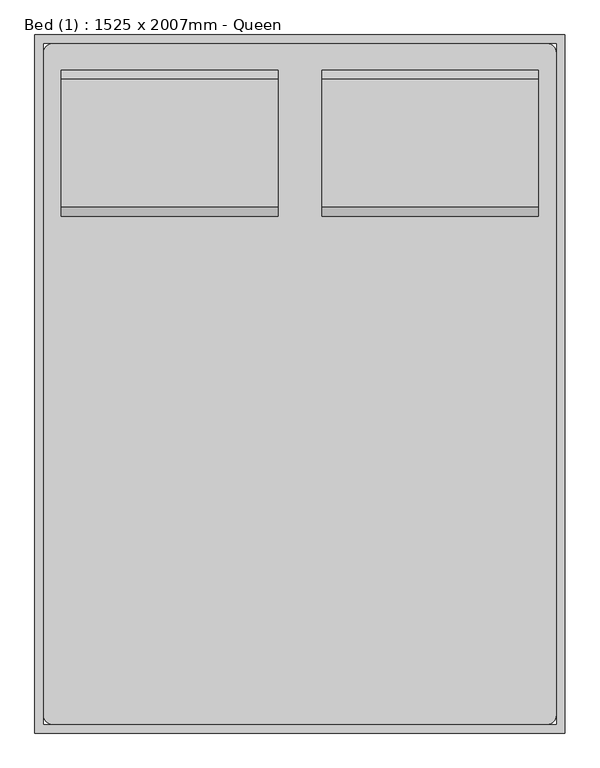
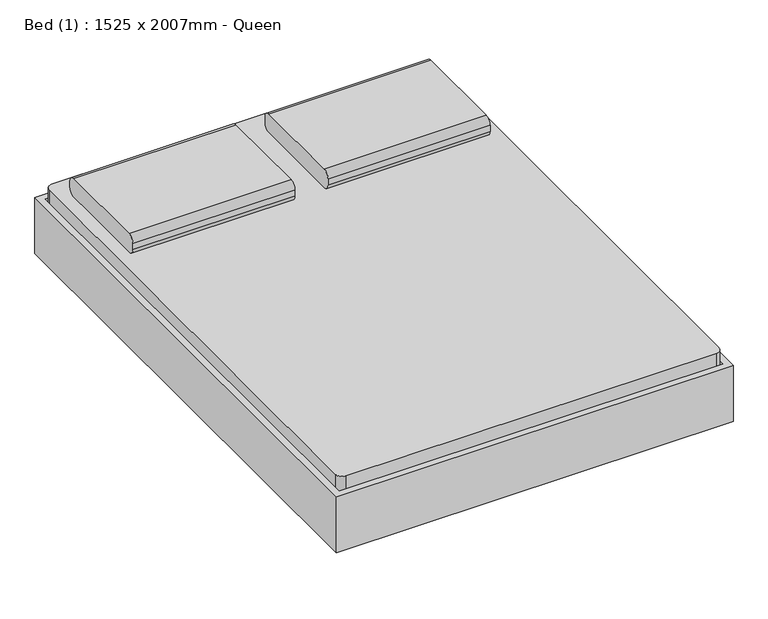
"""IFC4 building model written with IfcOpenShell, lengths in millimetres: furniture geometry, Bed (1) : 1525 x 2007mm - Queen."""

from ifc_helpers import new_model, si_unit, point, frame, frame_2d, origin, place, context, project, spatial, polyline, circle_curve, trimmed, segment, composite_curve, outline, extrude, source, transform, mapped, element, save
from ifc_brep_helpers import plane_surface, cylinder_surface, revolved_surface, advanced_brep


def bed_1_1525_x_2007mm_queen_eef227c3(model_context):
    return source(origin(), model_context, "Body", "SolidModel", [
        advanced_brep(
        [(-397.947541, -933.1295082, 196.85), (-397.947541, -933.1295082, 177.8), (-397.947541, -1009.3295082, 177.8), (-397.947541, -1009.3295082, 196.85), (-335.0113525, -933.1295082, 196.85), (-347.147541, -933.1295082, 177.8), (-347.147541, -1009.3295082, 177.8), (-335.0113525, -1009.3295082, 196.85), (-253.8115092, -933.1295082, 22.716374), (-271.0766725, -933.1295082, 14.6654962), (-271.0766725, -1009.3295082, 14.6654962), (-253.8115092, -1009.3295082, 22.716374), (-248.0564547, -933.1295082, 0.0), (-248.0564547, -933.1295082, 19.05), (-248.0564547, -1009.3295082, 0.0), (-248.0564547, -1009.3295082, 19.05), (-169.4439489, -933.1295082, 19.05), (-169.4439489, -933.1295082, 0.0), (-169.4439489, -1009.3295082, 0.0), (-169.4439489, -1009.3295082, 19.05), (-156.7439489, -933.1295082, 3.4029547), (-166.2689489, -933.1295082, 19.9007387), (-156.7439489, -1009.3295082, 3.4029547), (-166.2689489, -1009.3295082, 19.9007387), (-101.7513357, -933.1295082, 57.15), (-96.6469036, -933.1295082, 38.1), (-96.6469036, -1009.3295082, 38.1), (-101.7513357, -1009.3295082, 57.15), (780.0562537, -933.1295082, 57.15), (774.9518216, -933.1295082, 38.1), (774.9518216, -1009.3295082, 38.1), (780.0562537, -1009.3295082, 57.15), (844.5738669, -933.1295082, 19.9007387), (835.0488669, -933.1295082, 3.4029547), (835.0488669, -1009.3295082, 3.4029547), (844.5738669, -1009.3295082, 19.9007387), (847.7488669, -933.1295082, 0.0), (847.7488669, -933.1295082, 19.05), (847.7488669, -1009.3295082, 0.0), (847.7488669, -1009.3295082, 19.05), (926.3613728, -933.1295082, 19.05), (926.3613728, -933.1295082, 0.0), (926.3613728, -1009.3295082, 0.0), (926.3613728, -1009.3295082, 19.05), (949.3815906, -933.1295082, 14.6654962), (932.1164272, -933.1295082, 22.716374), (949.3815906, -1009.3295082, 14.6654962), (932.1164272, -1009.3295082, 22.716374), (1013.3162705, -933.1295082, 196.85), (1025.452459, -933.1295082, 177.8), (1025.452459, -1009.3295082, 177.8), (1013.3162705, -1009.3295082, 196.85), (1076.252459, -933.1295082, 196.85), (1076.252459, -1009.3295082, 196.85), (1076.252459, -1009.3295082, 177.8), (1076.252459, -933.1295082, 177.8)],
        [
            (0, 1),
            (1, 2),
            (2, 3),
            (3, 0),
            (0, 4),
            (4, 5),
            (5, 1),
            (5, 6),
            (6, 2),
            (6, 7),
            (7, 3),
            (7, 4),
            (4, 8),
            (8, 9),
            (9, 5),
            (9, 10),
            (10, 6),
            (10, 11),
            (11, 7),
            (11, 8),
            (12, 9, circle_curve(frame((-248.0564547, -933.1295082, 25.4), z_axis=(0.0, 1.0, 0.0), x_axis=(-0.906307787036664, 0.0, -0.4226182617406693)), 25.4)),
            (8, 13, circle_curve(frame((-248.0564547, -933.1295082, 25.4), z_axis=(0.0, -1.0, 0.0), x_axis=(-0.906307787036664, 0.0, -0.4226182617406693)), 6.35)),
            (13, 12),
            (14, 10, circle_curve(frame((-248.0564547, -1009.3295082, 25.4), z_axis=(0.0, 1.0, 0.0), x_axis=(-0.906307787036664, 0.0, -0.4226182617406693)), 25.4)),
            (12, 14),
            (15, 11, circle_curve(frame((-248.0564547, -1009.3295082, 25.4), z_axis=(0.0, 1.0, 0.0), x_axis=(-0.906307787036664, 0.0, -0.4226182617406693)), 6.35)),
            (14, 15),
            (15, 13),
            (13, 16),
            (16, 17),
            (17, 12),
            (17, 18),
            (18, 14),
            (18, 19),
            (19, 15),
            (19, 16),
            (20, 17, circle_curve(frame((-169.4439489, -933.1295082, 25.4), z_axis=(0.0, 1.0, 0.0), x_axis=(0.0, 0.0, -1.0)), 25.4)),
            (16, 21, circle_curve(frame((-169.4439489, -933.1295082, 25.4), z_axis=(0.0, -1.0, 0.0), x_axis=(0.0, 0.0, -1.0)), 6.35)),
            (21, 20),
            (22, 18, circle_curve(frame((-169.4439489, -1009.3295082, 25.4), z_axis=(0.0, 1.0, 0.0), x_axis=(0.0, 0.0, -1.0)), 25.4)),
            (20, 22),
            (23, 19, circle_curve(frame((-169.4439489, -1009.3295082, 25.4), z_axis=(0.0, 1.0, 0.0), x_axis=(0.0, 0.0, -1.0)), 6.35)),
            (22, 23),
            (23, 21),
            (21, 24),
            (24, 25),
            (25, 20),
            (25, 26),
            (26, 22),
            (26, 27),
            (27, 23),
            (27, 24),
            (24, 28),
            (28, 29),
            (29, 25),
            (29, 30),
            (30, 26),
            (30, 31),
            (31, 27),
            (31, 28),
            (28, 32),
            (32, 33),
            (33, 29),
            (33, 34),
            (34, 30),
            (34, 35),
            (35, 31),
            (35, 32),
            (36, 33, circle_curve(frame((847.7488669, -933.1295082, 25.4), z_axis=(0.0, 1.0, 0.0), x_axis=(-0.5000000000000533, 0.0, -0.866025403784408)), 25.4)),
            (32, 37, circle_curve(frame((847.7488669, -933.1295082, 25.4), z_axis=(0.0, -1.0, 0.0), x_axis=(-0.5000000000000533, 0.0, -0.866025403784408)), 6.35)),
            (37, 36),
            (38, 34, circle_curve(frame((847.7488669, -1009.3295082, 25.4), z_axis=(0.0, 1.0, 0.0), x_axis=(-0.5000000000000533, 0.0, -0.866025403784408)), 25.4)),
            (36, 38),
            (39, 35, circle_curve(frame((847.7488669, -1009.3295082, 25.4), z_axis=(0.0, 1.0, 0.0), x_axis=(-0.5000000000000533, 0.0, -0.866025403784408)), 6.35)),
            (38, 39),
            (39, 37),
            (37, 40),
            (40, 41),
            (41, 36),
            (41, 42),
            (42, 38),
            (42, 43),
            (43, 39),
            (43, 40),
            (44, 41, circle_curve(frame((926.3613728, -933.1295082, 25.4), z_axis=(0.0, 1.0, 0.0), x_axis=(0.0, 0.0, -1.0)), 25.4)),
            (40, 45, circle_curve(frame((926.3613728, -933.1295082, 25.4), z_axis=(0.0, -1.0, 0.0), x_axis=(0.0, 0.0, -1.0)), 6.35)),
            (45, 44),
            (46, 42, circle_curve(frame((926.3613728, -1009.3295082, 25.4), z_axis=(0.0, 1.0, 0.0), x_axis=(0.0, 0.0, -1.0)), 25.4)),
            (44, 46),
            (47, 43, circle_curve(frame((926.3613728, -1009.3295082, 25.4), z_axis=(0.0, 1.0, 0.0), x_axis=(0.0, 0.0, -1.0)), 6.35)),
            (46, 47),
            (47, 45),
            (45, 48),
            (48, 49),
            (49, 44),
            (49, 50),
            (50, 46),
            (50, 51),
            (51, 47),
            (51, 48),
            (52, 53),
            (53, 54),
            (54, 55),
            (55, 52),
            (48, 52),
            (55, 49),
            (54, 50),
            (53, 51),
        ],
        [
            plane_surface(frame((-397.947541, -1237.9295082, -127.5947323), z_axis=(-1.0, 0.0, 0.0), x_axis=(0.0, 1.0, 0.0))),
            plane_surface(frame((-397.947541, -933.1295082, 196.85), z_axis=(0.0, 1.0, 0.0), x_axis=(1.0, 0.0, 0.0))),
            plane_surface(frame((-397.947541, -933.1295082, 177.8), z_axis=(0.0, 0.0, -1.0), x_axis=(1.0, 0.0, 0.0))),
            plane_surface(frame((-397.947541, -1009.3295082, 177.8), z_axis=(0.0, -1.0, 0.0), x_axis=(1.0, 0.0, 0.0))),
            plane_surface(frame((-397.947541, -1009.3295082, 196.85), z_axis=(0.0, 0.0, 1.0), x_axis=(1.0, 0.0, 0.0))),
            plane_surface(frame((-335.0113525, -933.1295082, 196.85), z_axis=(0.0, 1.0, 0.0), x_axis=(0.42261826174067163, 0.0, -0.9063077870366629))),
            plane_surface(frame((-347.147541, -933.1295082, 177.8), z_axis=(-0.906307787036663, 0.0, -0.4226182617406716), x_axis=(0.4226182617406716, 0.0, -0.906307787036663))),
            plane_surface(frame((-347.147541, -1009.3295082, 177.8), z_axis=(0.0, -1.0000000000000002, 0.0), x_axis=(0.4226182617406714, 0.0, -0.9063077870366631))),
            plane_surface(frame((-335.0113525, -1009.3295082, 196.85), z_axis=(0.906307787036663, 0.0, 0.4226182617406716), x_axis=(0.4226182617406716, 0.0, -0.906307787036663))),
            plane_surface(frame((-248.0564547, -933.1295082, 25.4), z_axis=(0.0, 1.0, 0.0), x_axis=(-0.906307787036664, 0.0, -0.4226182617406693))),
            cylinder_surface(frame((-248.0564547, -1237.9295082, 25.4), z_axis=(0.0, -1.0, 0.0), x_axis=(-0.906307787036664, 0.0, -0.4226182617406693)), 25.4),
            plane_surface(frame((-248.0564547, -1009.3295082, 25.4), z_axis=(0.0, -1.0, 0.0), x_axis=(-0.906307787036664, 0.0, -0.4226182617406693))),
            revolved_surface(polyline([(-253.8115091476828, -1009.3295082, 22.71637403794675), (-253.8115091476828, -933.1295082, 22.71637403794675)]), (-248.0564547, -1237.9295082, 25.4), (0.0, -1.0, 0.0)),
            plane_surface(frame((-248.0564547, -933.1295082, 19.05), z_axis=(0.0, 1.0, 0.0), x_axis=(1.0, 0.0, 0.0))),
            plane_surface(frame((-248.0564547, -933.1295082, 0.0), z_axis=(0.0, 0.0, -1.0), x_axis=(1.0, 0.0, 0.0))),
            plane_surface(frame((-248.0564547, -1009.3295082, 0.0), z_axis=(0.0, -1.0, 0.0), x_axis=(1.0, 0.0, 0.0))),
            plane_surface(frame((-248.0564547, -1009.3295082, 19.05), z_axis=(0.0, 0.0, 1.0), x_axis=(1.0, 0.0, 0.0))),
            plane_surface(frame((-169.4439489, -933.1295082, 25.4), z_axis=(0.0, 1.0, 0.0), x_axis=(0.0, 0.0, -1.0))),
            cylinder_surface(frame((-169.4439489, -1237.9295082, 25.4), z_axis=(0.0, -1.0, 0.0), x_axis=(0.0, 0.0, -1.0)), 25.4),
            plane_surface(frame((-169.4439489, -1009.3295082, 25.4), z_axis=(0.0, -1.0, 0.0), x_axis=(0.0, 0.0, -1.0))),
            revolved_surface(polyline([(-169.4439489, -1009.3295082, 19.049999999999997), (-169.4439489, -933.1295082, 19.049999999999997)]), (-169.4439489, -1237.9295082, 25.4), (0.0, -1.0, 0.0)),
            plane_surface(frame((-166.2689489, -933.1295082, 19.9007387), z_axis=(0.0, 1.0, 0.0), x_axis=(0.8660254037844783, 0.0, 0.4999999999999313))),
            plane_surface(frame((-156.7439489, -933.1295082, 3.4029547), z_axis=(0.499999999999931, 0.0, -0.8660254037844785), x_axis=(0.8660254037844785, 0.0, 0.499999999999931))),
            plane_surface(frame((-156.7439489, -1009.3295082, 3.4029547), z_axis=(0.0, -1.0, 0.0), x_axis=(0.8660254037844787, 0.0, 0.49999999999993067))),
            plane_surface(frame((-166.2689489, -1009.3295082, 19.9007387), z_axis=(-0.4999999999999307, 0.0, 0.8660254037844787), x_axis=(0.8660254037844787, 0.0, 0.4999999999999307))),
            plane_surface(frame((-101.7513357, -933.1295082, 57.15), z_axis=(0.0, 1.0, 0.0), x_axis=(1.0, 0.0, 0.0))),
            plane_surface(frame((-96.6469036, -933.1295082, 38.1), z_axis=(0.0, 0.0, -1.0), x_axis=(1.0, 0.0, 0.0))),
            plane_surface(frame((-96.6469036, -1009.3295082, 38.1), z_axis=(0.0, -1.0, 0.0), x_axis=(1.0, 0.0, 0.0))),
            plane_surface(frame((-101.7513357, -1009.3295082, 57.15), z_axis=(0.0, 0.0, 1.0), x_axis=(1.0, 0.0, 0.0))),
            plane_surface(frame((780.0562537, -933.1295082, 57.15), z_axis=(0.0, 1.0000000000000002, 0.0), x_axis=(0.8660254037844111, 0.0, -0.500000000000048))),
            plane_surface(frame((774.9518216, -933.1295082, 38.1), z_axis=(-0.5000000000000486, 0.0, -0.8660254037844106), x_axis=(0.8660254037844106, 0.0, -0.5000000000000486))),
            plane_surface(frame((774.9518216, -1009.3295082, 38.1), z_axis=(0.0, -1.0000000000000002, 0.0), x_axis=(0.8660254037844111, 0.0, -0.500000000000048))),
            plane_surface(frame((780.0562537, -1009.3295082, 57.15), z_axis=(0.5000000000000487, 0.0, 0.8660254037844106), x_axis=(0.8660254037844106, 0.0, -0.5000000000000487))),
            plane_surface(frame((847.7488669, -933.1295082, 25.4), z_axis=(0.0, 1.0, 0.0), x_axis=(-0.5000000000000533, 0.0, -0.866025403784408))),
            cylinder_surface(frame((847.7488669, -1237.9295082, 25.4), z_axis=(0.0, -1.0, 0.0), x_axis=(-0.5000000000000533, 0.0, -0.866025403784408)), 25.4),
            plane_surface(frame((847.7488669, -1009.3295082, 25.4), z_axis=(0.0, -1.0, 0.0), x_axis=(-0.5000000000000533, 0.0, -0.866025403784408))),
            revolved_surface(polyline([(844.5738668999998, -1009.3295082, 19.90073868596901), (844.5738668999998, -933.1295082, 19.90073868596901)]), (847.7488669, -1237.9295082, 25.4), (0.0, -1.0, 0.0)),
            plane_surface(frame((847.7488669, -933.1295082, 19.05), z_axis=(0.0, 1.0, 0.0), x_axis=(1.0, 0.0, 0.0))),
            plane_surface(frame((847.7488669, -933.1295082, 0.0), z_axis=(0.0, 0.0, -1.0), x_axis=(1.0, 0.0, 0.0))),
            plane_surface(frame((847.7488669, -1009.3295082, 0.0), z_axis=(0.0, -1.0, 0.0), x_axis=(1.0, 0.0, 0.0))),
            plane_surface(frame((847.7488669, -1009.3295082, 19.05), z_axis=(0.0, 0.0, 1.0), x_axis=(1.0, 0.0, 0.0))),
            plane_surface(frame((926.3613728, -933.1295082, 25.4), z_axis=(0.0, 1.0, 0.0), x_axis=(0.0, 0.0, -1.0))),
            cylinder_surface(frame((926.3613728, -1237.9295082, 25.4), z_axis=(0.0, -1.0, 0.0), x_axis=(0.0, 0.0, -1.0)), 25.4),
            plane_surface(frame((926.3613728, -1009.3295082, 25.4), z_axis=(0.0, -1.0, 0.0), x_axis=(0.0, 0.0, -1.0))),
            revolved_surface(polyline([(926.3613728, -1009.3295082, 19.049999999999997), (926.3613728, -933.1295082, 19.049999999999997)]), (926.3613728, -1237.9295082, 25.4), (0.0, -1.0, 0.0)),
            plane_surface(frame((932.1164272, -933.1295082, 22.716374), z_axis=(0.0, 1.0000000000000002, 0.0), x_axis=(0.4226182617405397, 0.0, 0.9063077870367245))),
            plane_surface(frame((949.3815906, -933.1295082, 14.6654962), z_axis=(0.9063077870367244, 0.0, -0.42261826174053974), x_axis=(0.42261826174053974, 0.0, 0.9063077870367244))),
            plane_surface(frame((949.3815906, -1009.3295082, 14.6654962), z_axis=(0.0, -1.0, 0.0), x_axis=(0.4226182617405396, 0.0, 0.9063077870367245))),
            plane_surface(frame((932.1164272, -1009.3295082, 22.716374), z_axis=(-0.9063077870367244, 0.0, 0.42261826174053996), x_axis=(0.42261826174053996, 0.0, 0.9063077870367244))),
            plane_surface(frame((1076.252459, -1237.9295082, -127.5947323), z_axis=(1.0, 0.0, 0.0), x_axis=(0.0, 1.0, 0.0))),
            plane_surface(frame((1013.3162705, -933.1295082, 196.85), z_axis=(0.0, 1.0, 0.0), x_axis=(1.0, 0.0, 0.0))),
            plane_surface(frame((1025.452459, -933.1295082, 177.8), z_axis=(0.0, 0.0, -1.0), x_axis=(1.0, 0.0, 0.0))),
            plane_surface(frame((1025.452459, -1009.3295082, 177.8), z_axis=(0.0, -1.0, 0.0), x_axis=(1.0, 0.0, 0.0))),
            plane_surface(frame((1013.3162705, -1009.3295082, 196.85), z_axis=(0.0, 0.0, 1.0), x_axis=(1.0, 0.0, 0.0))),
        ],
        [
            (0, [[1, 2, 3, 4]]),
            (1, [[-1, 5, 6, 7]]),
            (2, [[-2, -7, 8, 9]]),
            (3, [[-3, -9, 10, 11]]),
            (4, [[-4, -11, 12, -5]]),
            (5, [[-6, 13, 14, 15]]),
            (6, [[-8, -15, 16, 17]]),
            (7, [[-10, -17, 18, 19]]),
            (8, [[-12, -19, 20, -13]]),
            (9, [[21, -14, 22, 23]]),
            (10, [[24, -16, -21, 25]]),
            (11, [[26, -18, -24, 27]]),
            (12, [[-22, -20, -26, 28]]),
            (13, [[-23, 29, 30, 31]]),
            (14, [[-25, -31, 32, 33]]),
            (15, [[-27, -33, 34, 35]]),
            (16, [[-28, -35, 36, -29]]),
            (17, [[37, -30, 38, 39]]),
            (18, [[40, -32, -37, 41]]),
            (19, [[42, -34, -40, 43]]),
            (20, [[-38, -36, -42, 44]]),
            (21, [[-39, 45, 46, 47]]),
            (22, [[-41, -47, 48, 49]]),
            (23, [[-43, -49, 50, 51]]),
            (24, [[-44, -51, 52, -45]]),
            (25, [[-46, 53, 54, 55]]),
            (26, [[-48, -55, 56, 57]]),
            (27, [[-50, -57, 58, 59]]),
            (28, [[-52, -59, 60, -53]]),
            (29, [[-54, 61, 62, 63]]),
            (30, [[-56, -63, 64, 65]]),
            (31, [[-58, -65, 66, 67]]),
            (32, [[-60, -67, 68, -61]]),
            (33, [[69, -62, 70, 71]]),
            (34, [[72, -64, -69, 73]]),
            (35, [[74, -66, -72, 75]]),
            (36, [[-70, -68, -74, 76]]),
            (37, [[-71, 77, 78, 79]]),
            (38, [[-73, -79, 80, 81]]),
            (39, [[-75, -81, 82, 83]]),
            (40, [[-76, -83, 84, -77]]),
            (41, [[85, -78, 86, 87]]),
            (42, [[88, -80, -85, 89]]),
            (43, [[90, -82, -88, 91]]),
            (44, [[-86, -84, -90, 92]]),
            (45, [[-87, 93, 94, 95]]),
            (46, [[-89, -95, 96, 97]]),
            (47, [[-91, -97, 98, 99]]),
            (48, [[-92, -99, 100, -93]]),
            (49, [[101, 102, 103, 104]]),
            (50, [[-94, 105, -104, 106]]),
            (51, [[-96, -106, -103, 107]]),
            (52, [[-98, -107, -102, 108]]),
            (53, [[-100, -108, -101, -105]]),
        ],
    ),
        extrude(outline(composite_curve([segment(polyline([(-372.547541, 743.6704918), (1050.852459, 743.6704918)]), True, "CONTINUOUS"), segment(trimmed(circle_curve(frame_2d((1050.852459, 718.2704918)), 25.4), [point((1050.852459, 743.6704918))], [point((1076.252459, 718.2704918))], False, "CARTESIAN"), True, "CONTINUOUS"), segment(polyline([(1076.252459, 718.2704918), (1076.252459, -1187.1295082)]), True, "CONTINUOUS"), segment(trimmed(circle_curve(frame_2d((1050.852459, -1187.1295082)), 25.4), [point((1076.252459, -1187.1295082))], [point((1050.852459, -1212.5295082))], False, "CARTESIAN"), True, "CONTINUOUS"), segment(polyline([(1050.852459, -1212.5295082), (-372.547541, -1212.5295082)]), True, "CONTINUOUS"), segment(trimmed(circle_curve(frame_2d((-372.547541, -1187.1295082)), 25.4), [point((-372.547541, -1212.5295082))], [point((-397.947541, -1187.1295082))], False, "CARTESIAN"), True, "CONTINUOUS"), segment(polyline([(-397.947541, -1187.1295082), (-397.947541, 718.2704918)]), True, "CONTINUOUS"), segment(trimmed(circle_curve(frame_2d((-372.547541, 718.2704918)), 25.4), [point((-397.947541, 718.2704918))], [point((-372.547541, 743.6704918))], False, "CARTESIAN"), True, "CONTINUOUS")], self_intersect=False)), frame((0.0, 0.0, 203.2), z_axis=(0.0, 0.0, 1.0), x_axis=(1.0, 0.0, 0.0)), (0.0, 0.0, 1.0), 203.2),
        advanced_brep(
        [(-397.6231784, 515.0704918, 177.8), (-397.6231784, 438.8704918, 177.8), (-397.6231784, 438.8704918, 196.85), (-397.6231784, 515.0704918, 196.85), (-346.8231784, 515.0704918, 177.8), (-346.8231784, 438.8704918, 177.8), (-334.6869899, 438.8704918, 196.85), (-334.6869899, 515.0704918, 196.85), (-270.7523099, 515.0704918, 14.6654962), (-270.7523099, 438.8704918, 14.6654962), (-253.4871466, 438.8704918, 22.716374), (-253.4871466, 515.0704918, 22.716374), (-247.7320921, 438.8704918, 0.0), (-247.7320921, 515.0704918, 0.0), (-247.7320921, 438.8704918, 19.05), (-247.7320921, 515.0704918, 19.05), (-169.1195862, 515.0704918, 0.0), (-169.1195862, 438.8704918, 0.0), (-169.1195862, 438.8704918, 19.05), (-169.1195862, 515.0704918, 19.05), (-156.4195862, 438.8704918, 3.4029547), (-156.4195862, 515.0704918, 3.4029547), (-165.9445862, 438.8704918, 19.9007387), (-165.9445862, 515.0704918, 19.9007387), (-96.322541, 515.0704918, 38.1), (-96.322541, 438.8704918, 38.1), (-101.4269731, 438.8704918, 57.15), (-101.4269731, 515.0704918, 57.15), (774.9518216, 515.0704918, 38.1), (774.9518216, 438.8704918, 38.1), (780.0562537, 438.8704918, 57.15), (780.0562537, 515.0704918, 57.15), (835.0488669, 515.0704918, 3.4029547), (835.0488669, 438.8704918, 3.4029547), (844.5738669, 438.8704918, 19.9007387), (844.5738669, 515.0704918, 19.9007387), (847.7488669, 438.8704918, 0.0), (847.7488669, 515.0704918, 0.0), (847.7488669, 438.8704918, 19.05), (847.7488669, 515.0704918, 19.05), (926.3613728, 515.0704918, 0.0), (926.3613728, 438.8704918, 0.0), (926.3613728, 438.8704918, 19.05), (926.3613728, 515.0704918, 19.05), (949.3815906, 438.8704918, 14.6654962), (949.3815906, 515.0704918, 14.6654962), (932.1164272, 438.8704918, 22.716374), (932.1164272, 515.0704918, 22.716374), (1025.452459, 515.0704918, 177.8), (1025.452459, 438.8704918, 177.8), (1013.3162705, 438.8704918, 196.85), (1013.3162705, 515.0704918, 196.85), (1076.252459, 515.0704918, 177.8), (1076.252459, 515.0704918, 196.85), (1076.252459, 438.8704918, 196.85), (1076.252459, 438.8704918, 177.8)],
        [
            (0, 1),
            (1, 2),
            (2, 3),
            (3, 0),
            (0, 4),
            (4, 5),
            (5, 1),
            (5, 6),
            (6, 2),
            (6, 7),
            (7, 3),
            (7, 4),
            (4, 8),
            (8, 9),
            (9, 5),
            (9, 10),
            (10, 6),
            (10, 11),
            (11, 7),
            (11, 8),
            (12, 9, circle_curve(frame((-247.7320921, 438.8704918, 25.4), z_axis=(0.0, 1.0, 0.0), x_axis=(-0.906307787036649, 0.0, -0.4226182617407015)), 25.4)),
            (8, 13, circle_curve(frame((-247.7320921, 515.0704918, 25.4), z_axis=(0.0, -1.0, 0.0), x_axis=(-0.906307787036649, 0.0, -0.4226182617407015)), 25.4)),
            (13, 12),
            (14, 10, circle_curve(frame((-247.7320921, 438.8704918, 25.4), z_axis=(0.0, 1.0, 0.0), x_axis=(-0.906307787036649, 0.0, -0.4226182617407015)), 6.35)),
            (12, 14),
            (15, 11, circle_curve(frame((-247.7320921, 515.0704918, 25.4), z_axis=(0.0, 1.0, 0.0), x_axis=(-0.906307787036649, 0.0, -0.4226182617407015)), 6.35)),
            (14, 15),
            (15, 13),
            (13, 16),
            (16, 17),
            (17, 12),
            (17, 18),
            (18, 14),
            (18, 19),
            (19, 15),
            (19, 16),
            (20, 17, circle_curve(frame((-169.1195862, 438.8704918, 25.4), z_axis=(0.0, 1.0, 0.0), x_axis=(0.0, 0.0, -1.0)), 25.4)),
            (16, 21, circle_curve(frame((-169.1195862, 515.0704918, 25.4), z_axis=(0.0, -1.0, 0.0), x_axis=(0.0, 0.0, -1.0)), 25.4)),
            (21, 20),
            (22, 18, circle_curve(frame((-169.1195862, 438.8704918, 25.4), z_axis=(0.0, 1.0, 0.0), x_axis=(0.0, 0.0, -1.0)), 6.35)),
            (20, 22),
            (23, 19, circle_curve(frame((-169.1195862, 515.0704918, 25.4), z_axis=(0.0, 1.0, 0.0), x_axis=(0.0, 0.0, -1.0)), 6.35)),
            (22, 23),
            (23, 21),
            (21, 24),
            (24, 25),
            (25, 20),
            (25, 26),
            (26, 22),
            (26, 27),
            (27, 23),
            (27, 24),
            (24, 28),
            (28, 29),
            (29, 25),
            (29, 30),
            (30, 26),
            (30, 31),
            (31, 27),
            (31, 28),
            (28, 32),
            (32, 33),
            (33, 29),
            (33, 34),
            (34, 30),
            (34, 35),
            (35, 31),
            (35, 32),
            (36, 33, circle_curve(frame((847.7488669, 438.8704918, 25.4), z_axis=(0.0, 1.0, 0.0), x_axis=(-0.5000000000000449, 0.0, -0.8660254037844127)), 25.4)),
            (32, 37, circle_curve(frame((847.7488669, 515.0704918, 25.4), z_axis=(0.0, -1.0, 0.0), x_axis=(-0.5000000000000449, 0.0, -0.8660254037844127)), 25.4)),
            (37, 36),
            (38, 34, circle_curve(frame((847.7488669, 438.8704918, 25.4), z_axis=(0.0, 1.0, 0.0), x_axis=(-0.5000000000000449, 0.0, -0.8660254037844127)), 6.35)),
            (36, 38),
            (39, 35, circle_curve(frame((847.7488669, 515.0704918, 25.4), z_axis=(0.0, 1.0, 0.0), x_axis=(-0.5000000000000449, 0.0, -0.8660254037844127)), 6.35)),
            (38, 39),
            (39, 37),
            (37, 40),
            (40, 41),
            (41, 36),
            (41, 42),
            (42, 38),
            (42, 43),
            (43, 39),
            (43, 40),
            (44, 41, circle_curve(frame((926.3613728, 438.8704918, 25.4), z_axis=(0.0, 1.0, 0.0), x_axis=(0.0, 0.0, -1.0)), 25.4)),
            (40, 45, circle_curve(frame((926.3613728, 515.0704918, 25.4), z_axis=(0.0, -1.0, 0.0), x_axis=(0.0, 0.0, -1.0)), 25.4)),
            (45, 44),
            (46, 42, circle_curve(frame((926.3613728, 438.8704918, 25.4), z_axis=(0.0, 1.0, 0.0), x_axis=(0.0, 0.0, -1.0)), 6.35)),
            (44, 46),
            (47, 43, circle_curve(frame((926.3613728, 515.0704918, 25.4), z_axis=(0.0, 1.0, 0.0), x_axis=(0.0, 0.0, -1.0)), 6.35)),
            (46, 47),
            (47, 45),
            (45, 48),
            (48, 49),
            (49, 44),
            (49, 50),
            (50, 46),
            (50, 51),
            (51, 47),
            (51, 48),
            (52, 53),
            (53, 54),
            (54, 55),
            (55, 52),
            (48, 52),
            (55, 49),
            (54, 50),
            (53, 51),
        ],
        [
            plane_surface(frame((-397.6231784, 769.0704918, -152.9490627), z_axis=(-1.0, 0.0, 0.0), x_axis=(0.0, 1.0, 0.0))),
            plane_surface(frame((-397.6231784, 515.0704918, 177.8), z_axis=(0.0, 0.0, -1.0), x_axis=(1.0, 0.0, 0.0))),
            plane_surface(frame((-397.6231784, 438.8704918, 177.8), z_axis=(0.0, -1.0, 0.0), x_axis=(1.0, 0.0, 0.0))),
            plane_surface(frame((-397.6231784, 438.8704918, 196.85), z_axis=(0.0, 0.0, 1.0), x_axis=(1.0, 0.0, 0.0))),
            plane_surface(frame((-397.6231784, 515.0704918, 196.85), z_axis=(0.0, 1.0, 0.0), x_axis=(1.0, 0.0, 0.0))),
            plane_surface(frame((-346.8231784, 515.0704918, 177.8), z_axis=(-0.9063077870366485, 0.0, -0.4226182617407029), x_axis=(0.4226182617407029, 0.0, -0.9063077870366485))),
            plane_surface(frame((-346.8231784, 438.8704918, 177.8), z_axis=(0.0, -1.0, 0.0), x_axis=(0.42261826174070266, 0.0, -0.9063077870366485))),
            plane_surface(frame((-334.6869899, 438.8704918, 196.85), z_axis=(0.9063077870366486, 0.0, 0.4226182617407026), x_axis=(0.4226182617407026, 0.0, -0.9063077870366486))),
            plane_surface(frame((-334.6869899, 515.0704918, 196.85), z_axis=(0.0, 1.0, 0.0), x_axis=(0.42261826174070266, 0.0, -0.9063077870366485))),
            cylinder_surface(frame((-247.7320921, 769.0704918, 25.4), z_axis=(0.0, -1.0, 0.0), x_axis=(-0.906307787036649, 0.0, -0.4226182617407015)), 25.4),
            plane_surface(frame((-247.7320921, 438.8704918, 25.4), z_axis=(0.0, -1.0, 0.0), x_axis=(-0.906307787036649, 0.0, -0.4226182617407015))),
            revolved_surface(polyline([(-253.4871465476827, 438.8704918, 22.716374037946544), (-253.4871465476827, 515.0704918, 22.716374037946544)]), (-247.7320921, 769.0704918, 25.4), (0.0, -1.0, 0.0)),
            plane_surface(frame((-247.7320921, 515.0704918, 25.4), z_axis=(0.0, 1.0, 0.0), x_axis=(-0.906307787036649, 0.0, -0.4226182617407015))),
            plane_surface(frame((-247.7320921, 515.0704918, 0.0), z_axis=(0.0, 0.0, -1.0), x_axis=(1.0, 0.0, 0.0))),
            plane_surface(frame((-247.7320921, 438.8704918, 0.0), z_axis=(0.0, -1.0, 0.0), x_axis=(1.0, 0.0, 0.0))),
            plane_surface(frame((-247.7320921, 438.8704918, 19.05), z_axis=(0.0, 0.0, 1.0), x_axis=(1.0, 0.0, 0.0))),
            plane_surface(frame((-247.7320921, 515.0704918, 19.05), z_axis=(0.0, 1.0, 0.0), x_axis=(1.0, 0.0, 0.0))),
            cylinder_surface(frame((-169.1195862, 769.0704918, 25.4), z_axis=(0.0, -1.0, 0.0), x_axis=(0.0, 0.0, -1.0)), 25.4),
            plane_surface(frame((-169.1195862, 438.8704918, 25.4), z_axis=(0.0, -1.0, 0.0), x_axis=(0.0, 0.0, -1.0))),
            revolved_surface(polyline([(-169.1195862, 438.8704918, 19.049999999999997), (-169.1195862, 515.0704918, 19.049999999999997)]), (-169.1195862, 769.0704918, 25.4), (0.0, -1.0, 0.0)),
            plane_surface(frame((-169.1195862, 515.0704918, 25.4), z_axis=(0.0, 1.0, 0.0), x_axis=(0.0, 0.0, -1.0))),
            plane_surface(frame((-156.4195862, 515.0704918, 3.4029547), z_axis=(0.49999999999987815, 0.0, -0.866025403784509), x_axis=(0.866025403784509, 0.0, 0.49999999999987815))),
            plane_surface(frame((-156.4195862, 438.8704918, 3.4029547), z_axis=(0.0, -1.0, 0.0), x_axis=(0.8660254037845089, 0.0, 0.49999999999987843))),
            plane_surface(frame((-165.9445862, 438.8704918, 19.9007387), z_axis=(-0.49999999999987776, 0.0, 0.8660254037845092), x_axis=(0.8660254037845092, 0.0, 0.49999999999987776))),
            plane_surface(frame((-165.9445862, 515.0704918, 19.9007387), z_axis=(0.0, 1.0, 0.0), x_axis=(0.8660254037845091, 0.0, 0.4999999999998781))),
            plane_surface(frame((-96.322541, 515.0704918, 38.1), z_axis=(0.0, 0.0, -1.0), x_axis=(1.0, 0.0, 0.0))),
            plane_surface(frame((-96.322541, 438.8704918, 38.1), z_axis=(0.0, -1.0, 0.0), x_axis=(1.0, 0.0, 0.0))),
            plane_surface(frame((-101.4269731, 438.8704918, 57.15), z_axis=(0.0, 0.0, 1.0), x_axis=(1.0, 0.0, 0.0))),
            plane_surface(frame((-101.4269731, 515.0704918, 57.15), z_axis=(0.0, 1.0, 0.0), x_axis=(1.0, 0.0, 0.0))),
            plane_surface(frame((774.9518216, 515.0704918, 38.1), z_axis=(-0.5000000000000465, 0.0, -0.8660254037844118), x_axis=(0.8660254037844118, 0.0, -0.5000000000000465))),
            plane_surface(frame((774.9518216, 438.8704918, 38.1), z_axis=(0.0, -1.0, 0.0), x_axis=(0.8660254037844123, 0.0, -0.5000000000000456))),
            plane_surface(frame((780.0562537, 438.8704918, 57.15), z_axis=(0.500000000000046, 0.0, 0.8660254037844122), x_axis=(0.8660254037844122, 0.0, -0.500000000000046))),
            plane_surface(frame((780.0562537, 515.0704918, 57.15), z_axis=(0.0, 1.0, 0.0), x_axis=(0.8660254037844127, 0.0, -0.500000000000045))),
            cylinder_surface(frame((847.7488669, 769.0704918, 25.4), z_axis=(0.0, -1.0, 0.0), x_axis=(-0.5000000000000449, 0.0, -0.8660254037844127)), 25.4),
            plane_surface(frame((847.7488669, 438.8704918, 25.4), z_axis=(0.0, -1.0, 0.0), x_axis=(-0.5000000000000449, 0.0, -0.8660254037844127))),
            revolved_surface(polyline([(844.5738668999998, 438.8704918, 19.900738685968978), (844.5738668999998, 515.0704918, 19.900738685968978)]), (847.7488669, 769.0704918, 25.4), (0.0, -1.0, 0.0)),
            plane_surface(frame((847.7488669, 515.0704918, 25.4), z_axis=(0.0, 1.0, 0.0), x_axis=(-0.5000000000000449, 0.0, -0.8660254037844127))),
            plane_surface(frame((847.7488669, 515.0704918, 0.0), z_axis=(0.0, 0.0, -1.0), x_axis=(1.0, 0.0, 0.0))),
            plane_surface(frame((847.7488669, 438.8704918, 0.0), z_axis=(0.0, -1.0, 0.0), x_axis=(1.0, 0.0, 0.0))),
            plane_surface(frame((847.7488669, 438.8704918, 19.05), z_axis=(0.0, 0.0, 1.0), x_axis=(1.0, 0.0, 0.0))),
            plane_surface(frame((847.7488669, 515.0704918, 19.05), z_axis=(0.0, 1.0, 0.0), x_axis=(1.0, 0.0, 0.0))),
            cylinder_surface(frame((926.3613728, 769.0704918, 25.4), z_axis=(0.0, -1.0, 0.0), x_axis=(0.0, 0.0, -1.0)), 25.4),
            plane_surface(frame((926.3613728, 438.8704918, 25.4), z_axis=(0.0, -1.0, 0.0), x_axis=(0.0, 0.0, -1.0))),
            revolved_surface(polyline([(926.3613728, 438.8704918, 19.049999999999997), (926.3613728, 515.0704918, 19.049999999999997)]), (926.3613728, 769.0704918, 25.4), (0.0, -1.0, 0.0)),
            plane_surface(frame((926.3613728, 515.0704918, 25.4), z_axis=(0.0, 1.0, 0.0), x_axis=(0.0, 0.0, -1.0))),
            plane_surface(frame((949.3815906, 515.0704918, 14.6654962), z_axis=(0.9063077870366809, 0.0, -0.4226182617406331), x_axis=(0.4226182617406331, 0.0, 0.9063077870366809))),
            plane_surface(frame((949.3815906, 438.8704918, 14.6654962), z_axis=(0.0, -1.0000000000000002, 0.0), x_axis=(0.42261826174063377, 0.0, 0.9063077870366807))),
            plane_surface(frame((932.1164272, 438.8704918, 22.716374), z_axis=(-0.9063077870366809, 0.0, 0.42261826174063327), x_axis=(0.42261826174063327, 0.0, 0.9063077870366809))),
            plane_surface(frame((932.1164272, 515.0704918, 22.716374), z_axis=(0.0, 1.0, 0.0), x_axis=(0.4226182617406339, 0.0, 0.9063077870366806))),
            plane_surface(frame((1076.252459, 769.0704918, -152.9490627), z_axis=(1.0, 0.0, 0.0), x_axis=(0.0, 1.0, 0.0))),
            plane_surface(frame((1025.452459, 515.0704918, 177.8), z_axis=(0.0, 0.0, -1.0), x_axis=(1.0, 0.0, 0.0))),
            plane_surface(frame((1025.452459, 438.8704918, 177.8), z_axis=(0.0, -1.0, 0.0), x_axis=(1.0, 0.0, 0.0))),
            plane_surface(frame((1013.3162705, 438.8704918, 196.85), z_axis=(0.0, 0.0, 1.0), x_axis=(1.0, 0.0, 0.0))),
            plane_surface(frame((1013.3162705, 515.0704918, 196.85), z_axis=(0.0, 1.0, 0.0), x_axis=(1.0, 0.0, 0.0))),
        ],
        [
            (0, [[1, 2, 3, 4]]),
            (1, [[-1, 5, 6, 7]]),
            (2, [[-2, -7, 8, 9]]),
            (3, [[-3, -9, 10, 11]]),
            (4, [[-4, -11, 12, -5]]),
            (5, [[-6, 13, 14, 15]]),
            (6, [[-8, -15, 16, 17]]),
            (7, [[-10, -17, 18, 19]]),
            (8, [[-12, -19, 20, -13]]),
            (9, [[21, -14, 22, 23]]),
            (10, [[24, -16, -21, 25]]),
            (11, [[26, -18, -24, 27]]),
            (12, [[-22, -20, -26, 28]]),
            (13, [[-23, 29, 30, 31]]),
            (14, [[-25, -31, 32, 33]]),
            (15, [[-27, -33, 34, 35]]),
            (16, [[-28, -35, 36, -29]]),
            (17, [[37, -30, 38, 39]]),
            (18, [[40, -32, -37, 41]]),
            (19, [[42, -34, -40, 43]]),
            (20, [[-38, -36, -42, 44]]),
            (21, [[-39, 45, 46, 47]]),
            (22, [[-41, -47, 48, 49]]),
            (23, [[-43, -49, 50, 51]]),
            (24, [[-44, -51, 52, -45]]),
            (25, [[-46, 53, 54, 55]]),
            (26, [[-48, -55, 56, 57]]),
            (27, [[-50, -57, 58, 59]]),
            (28, [[-52, -59, 60, -53]]),
            (29, [[-54, 61, 62, 63]]),
            (30, [[-56, -63, 64, 65]]),
            (31, [[-58, -65, 66, 67]]),
            (32, [[-60, -67, 68, -61]]),
            (33, [[69, -62, 70, 71]]),
            (34, [[72, -64, -69, 73]]),
            (35, [[74, -66, -72, 75]]),
            (36, [[-70, -68, -74, 76]]),
            (37, [[-71, 77, 78, 79]]),
            (38, [[-73, -79, 80, 81]]),
            (39, [[-75, -81, 82, 83]]),
            (40, [[-76, -83, 84, -77]]),
            (41, [[85, -78, 86, 87]]),
            (42, [[88, -80, -85, 89]]),
            (43, [[90, -82, -88, 91]]),
            (44, [[-86, -84, -90, 92]]),
            (45, [[-87, 93, 94, 95]]),
            (46, [[-89, -95, 96, 97]]),
            (47, [[-91, -97, 98, 99]]),
            (48, [[-92, -99, 100, -93]]),
            (49, [[101, 102, 103, 104]]),
            (50, [[-94, 105, -104, 106]]),
            (51, [[-96, -106, -103, 107]]),
            (52, [[-98, -107, -102, 108]]),
            (53, [[-100, -108, -101, -105]]),
        ],
    ),
        extrude(outline(composite_curve([segment(polyline([(642.0704918, 406.4), (273.7704918, 406.4)]), True, "CONTINUOUS"), segment(trimmed(circle_curve(frame_2d((273.7704918, 431.8)), 25.4), [point((273.7704918, 406.4))], [point((248.3704918, 431.8))], False, "CARTESIAN"), True, "CONTINUOUS"), segment(polyline([(248.3704918, 431.8), (248.3704918, 457.2)]), True, "CONTINUOUS"), segment(trimmed(circle_curve(frame_2d((273.7704918, 457.2)), 25.4), [point((248.3704918, 457.2))], [point((273.7704918, 482.6))], False, "CARTESIAN"), True, "CONTINUOUS"), segment(polyline([(273.7704918, 482.6), (642.0704918, 482.6)]), True, "CONTINUOUS"), segment(trimmed(circle_curve(frame_2d((642.0704918, 457.2)), 25.4), [point((642.0704918, 482.6))], [point((667.4704918, 457.2))], False, "CARTESIAN"), True, "CONTINUOUS"), segment(polyline([(667.4704918, 457.2), (667.4704918, 431.8)]), True, "CONTINUOUS"), segment(trimmed(circle_curve(frame_2d((642.0704918, 431.8)), 25.4), [point((667.4704918, 431.8))], [point((642.0704918, 406.4))], False, "CARTESIAN"), True, "CONTINUOUS")], self_intersect=False)), frame((-347.147541, 0.0, 0.0), z_axis=(1.0, 0.0, 0.0), x_axis=(0.0, 1.0, 0.0)), (0.0, 0.0, 1.0), 622.8),
        extrude(outline(composite_curve([segment(polyline([(642.0704918, 406.4), (273.7704918, 406.4)]), True, "CONTINUOUS"), segment(trimmed(circle_curve(frame_2d((273.7704918, 431.8)), 25.4), [point((273.7704918, 406.4))], [point((248.3704918, 431.8))], False, "CARTESIAN"), True, "CONTINUOUS"), segment(polyline([(248.3704918, 431.8), (248.3704918, 457.2)]), True, "CONTINUOUS"), segment(trimmed(circle_curve(frame_2d((273.7704918, 457.2)), 25.4), [point((248.3704918, 457.2))], [point((273.7704918, 482.6))], False, "CARTESIAN"), True, "CONTINUOUS"), segment(polyline([(273.7704918, 482.6), (642.0704918, 482.6)]), True, "CONTINUOUS"), segment(trimmed(circle_curve(frame_2d((642.0704918, 457.2)), 25.4), [point((642.0704918, 482.6))], [point((667.4704918, 457.2))], False, "CARTESIAN"), True, "CONTINUOUS"), segment(polyline([(667.4704918, 457.2), (667.4704918, 431.8)]), True, "CONTINUOUS"), segment(trimmed(circle_curve(frame_2d((642.0704918, 431.8)), 25.4), [point((667.4704918, 431.8))], [point((642.0704918, 406.4))], False, "CARTESIAN"), True, "CONTINUOUS")], self_intersect=False)), frame((402.652459, 0.0, 0.0), z_axis=(1.0, 0.0, 0.0), x_axis=(0.0, 1.0, 0.0)), (0.0, 0.0, 1.0), 622.8),
        extrude(outline(polyline([(1101.652459, 769.0704918), (1101.652459, -1237.9295082), (-423.347541, -1237.9295082), (-423.347541, 769.0704918), (1101.652459, 769.0704918)]), holes=[polyline([(1076.252459, 743.6704918), (-397.947541, 743.6704918), (-397.947541, -1212.5295082), (1076.252459, -1212.5295082), (1076.252459, 743.6704918)])]), frame((0.0, 0.0, 127.0), z_axis=(0.0, 0.0, 1.0), x_axis=(1.0, 0.0, 0.0)), (0.0, 0.0, 1.0), 228.6),
    ])


if __name__ == "__main__":
    model = new_model("IFC4")
    model_context = context("Model", 3, world=origin())
    ifc_project = project(units=[si_unit("LENGTHUNIT", "METRE", prefix="MILLI")], contexts=[model_context])
    site = spatial("IfcSite", under=ifc_project)
    building = spatial("IfcBuilding", under=site)
    placement = place(None, origin())
    bed_1_1525_x_2007mm_queen_shape = bed_1_1525_x_2007mm_queen_eef227c3(model_context)
    element("IfcFurniture", 1, ObjectType="Bed (1) : 1525 x 2007mm - Queen", at=placement, inside=building, context=model_context, shape_type="MappedRepresentation", body=[
        mapped(bed_1_1525_x_2007mm_queen_shape, transform((0.0, 0.0, 0.0), x_axis=(1.0, 0.0, 0.0), y_axis=(0.0, 1.0, 0.0), z_axis=(0.0, 0.0, 1.0))),
    ])
    save(model, "model.ifc")

# Revit data of these elements
# Type "Bed (1) : 1525 x 2007mm - Queen"
#   Keynote = "N"
#   Length = 6' - 7.01575"
#   Width = 5' - 0.03937"
#   Material Frame = Wood - Birch
#   Material Mattress = Textile - White
#   Default Elevation = 0
# Element 1 (IfcFurniture, "Bed (1) : 1525 x 2007mm - Queen")
#   Materials on its faces: "Wood - Birch", "Textile - White"
# Materials
#   "Wood - Birch": colour RGB 224 178 126, transparency 0
#   "Textile - White": colour RGB 247 247 239, transparency 0
